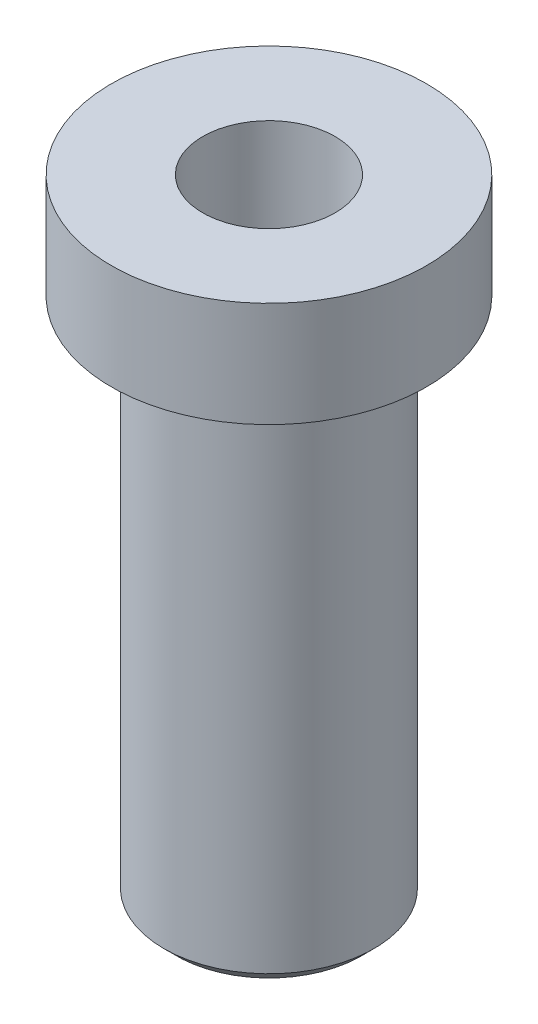
from build123d import *

# Parameters (mm, degrees)
SHANK_END_CHAMFER_6X45_SIZE = 6


with BuildPart() as part:
    # Pin Profile Sketch → Pin Body Revolve (revolve)
    with BuildSketch(Plane.XY, mode=Mode.PRIVATE) as pin_body_revolve_sk:
        Polygon((50, 0), (50, 250), (75, 250), (75, 300), (31.5, 300), (31.5, 0), align=None)
    revolve(pin_body_revolve_sk.sketch.rotate(Axis((0, 0, 0), (0, 1, 0)), 90), axis=Axis((0, 0, 0), (0, 1, 0)))

    # Shank End Chamfer 6x45°
    shank_end_chamfer_6x45_edges = [part.edges().sort_by_distance(p)[0] for p in [
        (0, 0, 50),
    ]]
    chamfer(shank_end_chamfer_6x45_edges, length=SHANK_END_CHAMFER_6X45_SIZE)


solid = part.part
